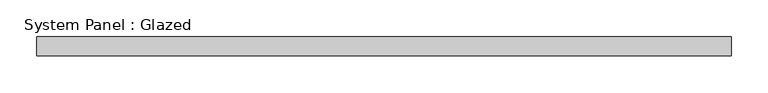
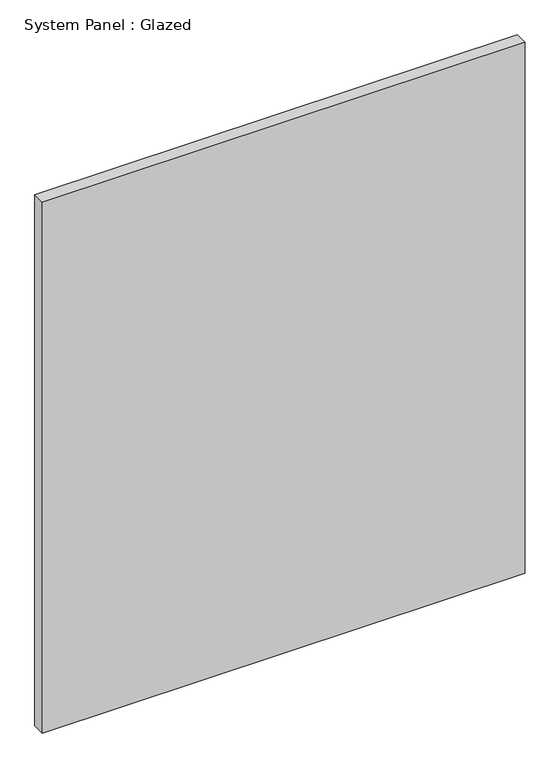
"""IFC4 building model written with IfcOpenShell, lengths in millimetres: plate geometry, System Panel : Glazed."""

from ifc_helpers import new_model, si_unit, origin, origin_with_axes, place, context, project, spatial, polyline, outline, extrude, source, transform, mapped, element, save


def system_panel_glazed_610bb4e0(model_context):
    return source(origin(), model_context, "Body", "SweptSolid", [
        extrude(outline(polyline([(469.9, 19.05), (-469.9, 19.05), (-469.9, 44.45), (469.9, 44.45), (469.9, 19.05)])), origin_with_axes(), (0.0, 0.0, 1.0), 1092.2),
    ])


if __name__ == "__main__":
    model = new_model("IFC4")
    model_context = context("Model", 3, world=origin())
    ifc_project = project(units=[si_unit("LENGTHUNIT", "METRE", prefix="MILLI")], contexts=[model_context])
    site = spatial("IfcSite", under=ifc_project)
    building = spatial("IfcBuilding", under=site)
    placement = place(None, origin())
    system_panel_glazed_shape = system_panel_glazed_610bb4e0(model_context)
    element("IfcPlate", 1, ObjectType="System Panel : Glazed", at=placement, inside=building, context=model_context, shape_type="MappedRepresentation", body=[
        mapped(system_panel_glazed_shape, transform((0.0, 0.0, 0.0), x_axis=(1.0, 0.0, 0.0), y_axis=(0.0, 1.0, 0.0), z_axis=(0.0, 0.0, 1.0))),
    ])
    save(model, "model.ifc")

# Revit data of these elements
# Type "System Panel : Glazed"
#   Construction Type Id = "GSP4R"
#   Analytic Construction = "1/8 in Pilkington single glazing"
#   Visual Light Transmittance = 0.9
#   Solar Heat Gain Coefficient = 0.86
#   Heat Transfer Coefficient (U) = 1.18115 BTU/(h·ft²·°F)
#   Define Thermal Properties by = 1
# Element 1 (IfcPlate, "System Panel : Glazed")
#   Materials on its faces: "Glass"
# Materials
#   "Glass": class "Glass", colour RGB 0 128 192, transparency 0.75, Description = "Soda Lime Glass", Cost = 0
